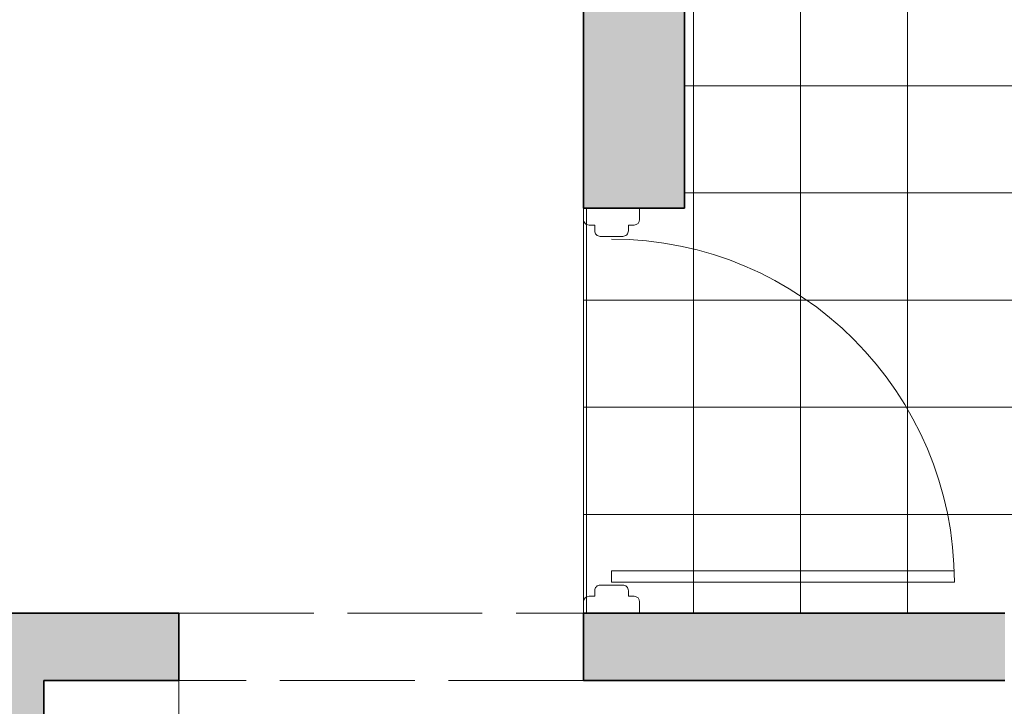
# Model space of a CAD drawing. Units: inches. Extents: x 84 to 1044, y -280 to 906.
# Tile 67 of 105: x 645 to 733, y 326 to 387. Entities that reach past the tile are written whole.
import ezdxf

# ---------------------------------------------------------------- set-up
doc = ezdxf.new("R2010")
doc.units = ezdxf.units.IN
doc.linetypes.add('ACAD_ISO02W100', pattern=[15, 12, -3])
for name, color, linetype, lineweight in [('00 FURNITURE', 15, 'Continuous', 15), ('A-DOOR', 4, 'Continuous', 18), ('A-FLOR-CASE', 8, 'Continuous', 18), ('A-WALL-OVHD', 8, 'ACAD_ISO02W100', 13), ('WALL', 250, 'Continuous', 35)]:
    doc.layers.add(name, color=color, linetype=linetype, lineweight=lineweight)
doc.layers.add('A-FLOR-PATT', color=251, linetype='Continuous', lineweight=9, true_color=0x705861)
doc.layers.add('A-WALL-PATT', color=251, linetype='Continuous', lineweight=9, true_color=0x636466)

# ---------------------------------------------------------------- blocks, each defined once
blk = doc.blocks.new('DDD')
at = {"layer": '00 FURNITURE'}
for p, q in [((-12579.773, -15859.529), (-12579.773, -15829.045)), ((-12578.773, -15859.529), (-12578.773, -15829.029)), ((-12612.023, -15857.029), (-12612.023, -15862.029)), ((-12611.023, -15857.029), (-12612.023, -15857.029)), ((-12577.023, -15857.029), (-12576.023, -15857.029)), ((-12576.023, -15857.029), (-12576.023, -15862.029)), ((-12610.523, -15858.029), (-12610.523, -15857.529)), ((-12577.523, -15858.029), (-12577.523, -15857.529)), ((-12578.773, -15859.529), (-12579.773, -15859.529)), ((-12610.523, -15861.529), (-12610.523, -15861.029)), ((-12577.523, -15861.529), (-12577.523, -15861.029)), ((-12612.023, -15862.029), (-12611.023, -15862.029)), ((-12576.023, -15862.029), (-12577.023, -15862.029))]:
    blk.add_line(p, q, dxfattribs=at)
for points in [[(-12610.523, -15861.029), (-12610.023, -15861.029, 0.414214), (-12609.523, -15860.529), (-12609.523, -15858.529, 0.414214), (-12610.023, -15858.029), (-12610.523, -15858.029)], [(-12577.523, -15861.029), (-12578.023, -15861.029, -0.414214), (-12578.523, -15860.529), (-12578.523, -15858.529, -0.414214), (-12578.023, -15858.029), (-12577.523, -15858.029)]]:
    blk.add_lwpolyline(points, format="xyb", dxfattribs=at)
for centre, radius, start, end in [((-12578.773, -15859.529), 30.5, 90, 180), ((-12611.023, -15857.529), 0.5, 0, 90), ((-12577.023, -15857.529), 0.5, 90, 180), ((-12611.023, -15861.529), 0.5, 270, 0), ((-12577.023, -15861.529), 0.5, 180, 270)]:
    blk.add_arc(centre, radius, start, end, dxfattribs=at)

msp = doc.modelspace()

# ---------------------------------------------------------------- hatches: boundary and pattern name
at = {"layer": 'A-FLOR-PATT', "transparency": 33554597}
h = msp.add_hatch(dxfattribs=at)
h.set_pattern_fill('ANSI37', color=256, scale=3, angle=45)
h.paths.add_polyline_path([(833.074, 388.12), (704.074, 388.12), (704.074, 370.12), (695.074, 370.12), (695.074, 334.12), (732.574, 334.12), (804.574, 334.12), (833.074, 334.12), (833.074, 364.12)])
at = {"layer": 'A-WALL-PATT', "transparency": 33554597}
h = msp.add_hatch(color=256, dxfattribs=at)
h.dxf.hatch_style = 1
h.paths.add_polyline_path([(671.074, 100.12), (647.074, 100.12), (647.074, 160.12), (641.074, 160.12), (620.824, 160.12), (620.824, 151.12), (638.074, 151.12), (638.074, 91.12), (671.074, 91.12)])
h.paths.add_polyline_path([(791.074, 100.12), (743.074, 100.12), (743.074, 91.12), (791.074, 91.12)])
h.paths.add_polyline_path([(896.074, 346.12), (887.074, 346.12), (887.074, 334.12), (870.955, 334.12), (833.074, 334.12), (804.574, 334.12), (804.574, 328.12), (887.074, 328.12), (887.074, 100.12), (863.074, 100.12), (863.074, 91.12), (896.074, 91.12)])
h.paths.add_polyline_path([(507.574, 154.729), (507.574, 160.12), (464.074, 160.12), (464.074, 247.12), (641.074, 247.12), (641.074, 208.12), (647.074, 208.12), (647.074, 328.12), (659.074, 328.12), (659.074, 334.12), (617.074, 334.12), (617.074, 328.12), (641.074, 328.12), (641.074, 256.12), (545.074, 256.12), (545.074, 328.12), (569.074, 328.12), (569.074, 334.12), (518.074, 334.12), (518.074, 325.12), (536.074, 325.12), (536.074, 256.12), (464.074, 256.12), (464.074, 325.12), (482.074, 325.12), (482.074, 334.12), (455.074, 334.12), (455.074, 160.12), (413.127, 160.12), (413.127, 151.12), (455.074, 151.12), (455.074, 91.12), (464.074, 91.12), (464.074, 151.12), (507.574, 151.12)])
h.paths.add_polyline_path([(572.824, 160.12), (555.574, 160.12), (555.574, 151.12), (572.824, 151.12)], flags=17)
h.paths.add_polyline_path([(341.127, 160.12), (299.179, 160.12), (299.179, 211.12), (294.179, 211.12), (290.179, 211.12), (290.179, 151.12), (341.127, 151.12)])
h.paths.add_polyline_path([(299.179, 256.12), (212.179, 256.12), (212.179, 274.12), (203.179, 274.12), (203.179, 247.12), (299.179, 247.12)])
h.paths.add_polyline_path([(212.179, 514.12), (398.074, 514.12), (398.074, 519.12), (398.074, 520.12), (212.179, 520.12), (212.179, 574.12), (203.179, 574.12), (203.179, 310.12), (212.179, 310.12), (212.179, 328.12), (290.179, 328.12), (290.179, 292.12), (299.179, 292.12), (299.179, 328.12), (332.179, 328.12), (332.179, 334.12), (212.179, 334.12)])
h.paths.add_polyline_path([(287.127, 709.12), (203.179, 709.12), (203.179, 646.12), (212.179, 646.12), (212.179, 700.12), (287.127, 700.12)])
h.paths.add_polyline_path([(470.074, 709.12), (359.127, 709.12), (359.127, 700.12), (434.074, 700.12), (434.074, 574.12), (440.074, 574.12), (440.074, 622.12), (464.074, 622.12), (464.074, 628.12), (440.074, 628.12), (440.074, 700.12), (470.074, 700.12)])
h.paths.add_polyline_path([(572.074, 709.12), (506.074, 709.12), (506.074, 700.12), (536.074, 700.12), (536.074, 628.12), (494.074, 628.12), (494.074, 622.12), (536.074, 622.12), (536.074, 520.12), (440.074, 520.12), (440.074, 544.12), (434.074, 544.12), (434.074, 514.12), (644.074, 514.12), (644.074, 519.12), (644.074, 544.12), (638.074, 544.12), (638.074, 520.12), (542.074, 520.12), (542.074, 622.12), (584.074, 622.12), (584.074, 628.12), (542.074, 628.12), (542.074, 700.12), (572.074, 700.12)])
h.paths.add_polyline_path([(698.074, 709.12), (608.074, 709.12), (608.074, 700.12), (638.074, 700.12), (638.074, 628.12), (614.074, 628.12), (614.074, 622.12), (638.074, 622.12), (638.074, 574.12), (644.074, 574.12), (644.074, 700.12), (698.074, 700.12)])
h.paths.add_polyline_path([(833.074, 709.12), (770.074, 709.12), (770.074, 700.12), (824.074, 700.12), (824.074, 646.12), (833.074, 646.12)])
h.paths.add_polyline_path([(833.074, 574.12), (824.074, 574.12), (824.074, 520.12), (791.244, 520.12), (712.904, 520.12), (680.074, 520.12), (680.074, 514.12), (695.074, 514.12), (695.074, 491.62), (704.074, 491.62), (704.074, 511.12), (833.074, 511.12)])
h.paths.add_polyline_path([(704.074, 419.62), (695.074, 419.62), (695.074, 370.12), (704.074, 370.12)])
h.paths.add_polyline_path([(896.074, 400.12), (833.074, 400.12), (833.074, 364.12), (839.074, 364.12), (839.074, 394.12), (887.074, 394.12), (887.074, 382.12), (896.074, 382.12)])
h.paths.add_polyline_path([(732.574, 334.12), (695.074, 334.12), (695.074, 328.12), (732.574, 328.12)])

# ---------------------------------------------------------------- linework, layer by layer
at = {"layer": 'A-DOOR'}
msp.add_line((695.074, 370.12), (695.074, 334.12), dxfattribs=at)
at = {"layer": 'A-FLOR-CASE'}
msp.add_line((659.074, 328.12), (659.074, 208.12), dxfattribs=at)
at = {"layer": 'A-WALL-OVHD'}
msp.add_lwpolyline([(695.074, 328.12), (659.074, 328.12), (659.074, 334.12), (695.074, 334.12)], close=True, dxfattribs=at)
at = {"layer": 'WALL'}
for p, q in [((695.074, 370.12), (695.074, 419.62)), ((704.074, 370.12), (704.074, 419.62)), ((704.074, 370.12), (695.074, 370.12)), ((659.074, 334.12), (617.074, 334.12)), ((659.074, 334.12), (659.074, 328.12)), ((695.074, 328.12), (695.074, 334.12)), ((732.574, 334.12), (695.074, 334.12)), ((647.074, 328.12), (647.074, 208.12)), ((659.074, 328.12), (647.074, 328.12)), ((732.574, 328.12), (695.074, 328.12))]:
    msp.add_line(p, q, dxfattribs=at)

# ---------------------------------------------------------------- block references
at = {"layer": 'A-DOOR', "rotation": 270}
msp.add_blockref('DDD', (16557.103, -12241.903), dxfattribs=at)

doc.saveas('drawing.dxf')
